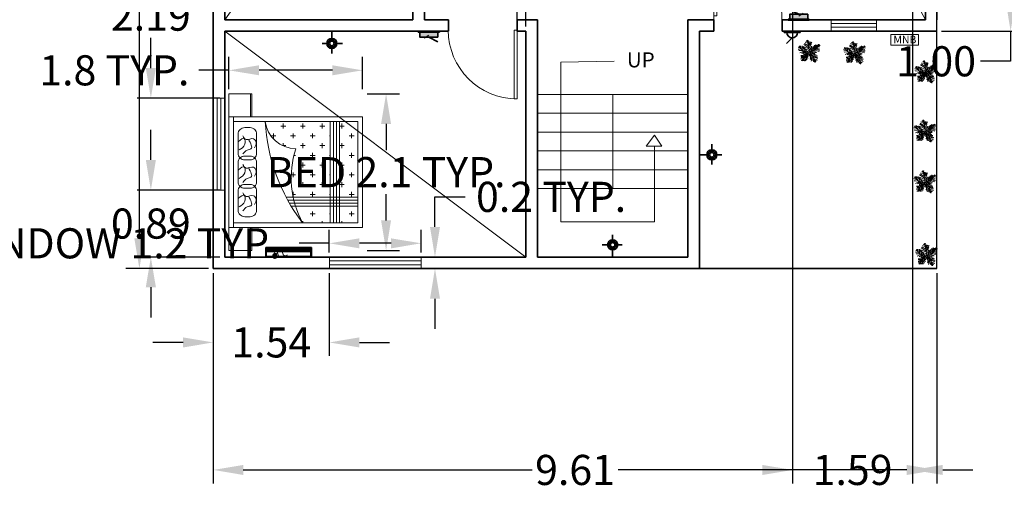
# Model space of a CAD drawing. Units: metres. Extents: x 24.2 to 58.5, y -14.5 to 15.2.
# Tile 4 of 7: x 38.9 to 51.9, y -1 to 5.2. Entities that reach past the tile are written whole.
import ezdxf

# ---------------------------------------------------------------- set-up
doc = ezdxf.new("R2010")
doc.units = ezdxf.units.M
doc.header["$MEASUREMENT"] = 0
for name, color, linetype, lineweight in [('A-ANNO-SYMB', 90, 'Continuous', 18), ('A-ANNO-TEXT', 10, 'Continuous', 18), ('A-FLOR', 7, 'Continuous', 25), ('A-FLOR-STRS', 7, 'Continuous', 18), ('A-GLAZ', 15, 'Continuous', 18), ('A-WALL', 7, 'Continuous', 35), ('DIMENSION', 90, 'Continuous', 18), ('DOOR', 15, 'Continuous', 18), ('E-COMM', 1, 'Continuous', 18), ('E-EQPM-LAYO', 1, 'Continuous', 13), ('E-LITE', 1, 'Continuous', 18), ('E-POWR', 1, 'Continuous', 18), ('E-POWR-EQPM', 1, 'Continuous', 18), ('Elec', 1, 'Continuous', 35), ('FURN', 163, 'Continuous', 13), ('L-PLNT', 90, 'Continuous', 13)]:
    doc.layers.add(name, color=color, linetype=linetype, lineweight=lineweight)
doc.styles.get("Standard").update_dxf_attribs({"font": 'arial.ttf'})
doc.dimstyles.get("Standard").update_dxf_attribs({"dimtxt": 0.4, "dimasz": 0.4, "dimexe": 0.18, "dimexo": 0.0625, "dimgap": 0.09, "dimtad": 0, "dimtih": 1, "dimtoh": 1, "dimdec": 1, "dimzin": 0, "dimdsep": 46, "dimtxsty": 'Standard', "dimcen": 0.09, "dimadec": 0, "dimazin": 0, "dimtfac": 1, "dimtdec": 1, "dimtofl": 0, "dimtmove": 0, "dimatfit": 3, "dimfxl": 1, "dimtolj": 1, "dimtzin": 0, "dimarcsym": 0})

# ---------------------------------------------------------------- blocks, each defined once
blk = doc.blocks.new('*U17')
for p, q in [((0, 0), (0, -6)), ((40, 0), (40, -6))]:
    blk.add_line(p, q)
blk.add_lwpolyline([(0, 0), (0, 40), (1.75, 40), (1.75, 0)], close=True)
blk.add_arc((0, 0), 40, 0, 90)
blk = doc.blocks.new('bed 1')
at = {"layer": 'FURN'}
h = blk.add_hatch(dxfattribs=at)
h.set_pattern_fill('CROSS', color=256, style=0)
h.set_pattern_definition([(0, (0, 0), (6.35, 6.35), [3.175, -9.525]), (90, (1.5875, -1.5875), (-6.35, 6.35), [3.175, -9.525])])
h.paths.add_polyline_path([(1334.16, -843.32, 0.37496), (1316.43, -863.27, 0.131129), (1284.95, -861.51), (1284.95, -885.72), (1334.16, -885.72)])
h.paths.add_polyline_path([(1278.95, -863.08, 0.048033), (1268.16, -867.67), (1268.16, -885.72), (1278.95, -885.72)])
h.paths.add_polyline_path([(1278.95, -891.72), (1268.16, -891.72), (1268.16, -903.72), (1278.95, -903.72)])
h.paths.add_polyline_path([(1334.16, -891.72), (1284.95, -891.72), (1284.95, -903.72), (1334.16, -903.72)])
for p, q in [((1265.16, -819.72), (1250.16, -819.72)), ((1250.16, -819.72), (1250.16, -834.72)), ((1337.16, -819.72), (1265.16, -819.72)), ((1265.16, -819.72), (1265.16, -906.72)), ((1337.16, -906.72), (1337.16, -819.72)), ((1337.16, -819.72), (1352.16, -819.72)), ((1352.16, -819.72), (1352.16, -834.72)), ((1337.16, -822.72), (1265.16, -822.72)), ((1268.16, -822.72), (1268.16, -903.72)), ((1334.16, -903.72), (1334.16, -822.72)), ((1250.16, -833.72), (1265.16, -833.72)), ((1250.16, -834.72), (1265.16, -834.72)), ((1352.16, -833.72), (1337.16, -833.72)), ((1352.16, -834.72), (1337.16, -834.72)), ((1282.95, -903.72), (1282.95, -857.98)), ((1284.95, -903.72), (1284.95, -856.89)), ((1278.95, -903.72), (1278.95, -860.29)), ((1280.95, -903.72), (1280.95, -859.11)), ((1334.16, -885.72), (1268.16, -885.72)), ((1334.16, -887.72), (1268.16, -887.72)), ((1334.16, -889.72), (1268.16, -889.72)), ((1334.16, -891.72), (1268.16, -891.72)), ((1268.16, -903.72), (1334.16, -903.72)), ((1265.16, -906.72), (1337.16, -906.72))]:
    blk.add_line(p, q, dxfattribs=at)
for points in [[(1288.91, -837.72), (1276.42, -837.72, -0.414214), (1272.16, -833.47), (1272.16, -829.98, -0.414214), (1276.42, -825.72), (1288.91, -825.72, -0.414214), (1293.16, -829.98), (1293.16, -833.47, -0.414214)], [(1307.41, -837.72), (1294.92, -837.72, -0.414214), (1290.66, -833.47), (1290.66, -829.98, -0.414214), (1294.92, -825.72), (1307.41, -825.72, -0.414214), (1311.66, -829.98), (1311.66, -833.47, -0.414214)], [(1325.91, -837.72), (1313.42, -837.72, -0.414214), (1309.16, -833.47), (1309.16, -829.98, -0.414214), (1313.42, -825.72), (1325.91, -825.72, -0.414214), (1330.16, -829.98), (1330.16, -833.47, -0.414214)], [(1334.16, -843.32, 0.151933), (1268.16, -867.67), (1268.16, -867.67, -0.20661), (1316.43, -863.27), (1316.43, -863.27, -0.37496)]]:
    blk.add_lwpolyline(points, format="xyb", close=True, dxfattribs=at)
for points, knots in [([(1278.62, -826.37), (1279.52, -827.92), (1281.07, -830.61), (1287.77, -830.3), (1285.41, -827.44), (1284.17, -825.93)], [0, 0, 0, 0, 4.23607, 7.317462, 10.761159, 10.761159, 10.761159, 10.761159]), ([(1297.12, -826.37), (1298.02, -827.92), (1299.57, -830.61), (1306.27, -830.3), (1303.91, -827.44), (1302.67, -825.93)], [0, 0, 0, 0, 4.23607, 7.317462, 10.761159, 10.761159, 10.761159, 10.761159]), ([(1315.62, -826.37), (1316.52, -827.92), (1318.07, -830.61), (1324.77, -830.3), (1322.41, -827.44), (1321.17, -825.93)], [0, 0, 0, 0, 4.23607, 7.317462, 10.761159, 10.761159, 10.761159, 10.761159]), ([(1275.98, -828.74), (1277, -829.54), (1278.71, -830.85), (1279.22, -835.95), (1282.92, -833.91), (1285.58, -832.44)], [0, 0, 0, 0, 3.079719, 5.108686, 10.317752, 10.317752, 10.317752, 10.317752]), ([(1287.7, -828.74), (1286.63, -829.38), (1283.96, -830.98), (1287.28, -835.52), (1283.18, -838.02), (1281.17, -836.99), (1280.03, -836.4)], [0, 0, 0, 0, 2.624379, 6.568207, 8.823918, 11.783788, 11.783788, 11.783788, 11.783788]), ([(1294.48, -828.74), (1295.5, -829.54), (1297.21, -830.85), (1297.72, -835.95), (1301.42, -833.91), (1304.08, -832.44)], [0, 0, 0, 0, 3.079719, 5.108686, 10.317752, 10.317752, 10.317752, 10.317752]), ([(1306.2, -828.74), (1305.13, -829.38), (1302.46, -830.98), (1305.78, -835.52), (1301.68, -838.02), (1299.67, -836.99), (1298.53, -836.4)], [0, 0, 0, 0, 2.624379, 6.568207, 8.823918, 11.783788, 11.783788, 11.783788, 11.783788]), ([(1312.98, -828.74), (1314, -829.54), (1315.71, -830.85), (1316.22, -835.95), (1319.92, -833.91), (1322.58, -832.44)], [0, 0, 0, 0, 3.079719, 5.108686, 10.317752, 10.317752, 10.317752, 10.317752]), ([(1324.7, -828.74), (1323.63, -829.38), (1320.96, -830.98), (1324.28, -835.52), (1320.18, -838.02), (1318.17, -836.99), (1317.03, -836.4)], [0, 0, 0, 0, 2.624379, 6.568207, 8.823918, 11.783788, 11.783788, 11.783788, 11.783788])]:
    blk.add_open_spline(points, degree=3, knots=knots, dxfattribs=at)
blk = doc.blocks.new('splight')
at = {"layer": 'Elec'}
for p, q in [((4618.17, 527.16), (4627.57, 527.16)), ((4622.87, 527.16), (4622.87, 523.87)), ((4620.58, 521.58), (4618.05, 521.58)), ((4625.16, 521.58), (4627.23, 521.58)), ((4622.87, 519.28), (4622.87, 517.03))]:
    blk.add_line(p, q, dxfattribs=at)
for radius in [2.29, 1.67, 1.04]:
    blk.add_circle((4622.87, 521.58), radius, dxfattribs=at)
blk = doc.blocks.new('BELL SWITCH')
at = {"layer": 'Elec'}
for p, q in [((4981.81, 3401.31), (4981.81, 3402.27)), ((4981.81, 3402.27), (4993.57, 3402.27)), ((4993.57, 3401.31), (4981.81, 3401.31)), ((4987.69, 3397.36), (4983.52, 3393.3)), ((4993.57, 3402.27), (4993.57, 3401.31))]:
    blk.add_line(p, q, dxfattribs=at)
blk.add_arc((4987.69, 3401.31), 3.95, 180, 0, dxfattribs=at)
blk = doc.blocks.new('*U44')
for p, q in [((-8.737, 47.138), (-17.069, 52.711)), ((-10.186, 53.64), (-13.084, 55.962)), ((0, 0), (-10.5, 57)), ((-9.099, 51.782), (-6.563, 55.962)), ((-7.65, 43.423), (-2.578, 49.46)), ((-5.839, 35.992), (4.667, 48.067)), ((-47.498, 19.737), (-55.83, 18.344)), ((-40.615, 13.7), (-55.105, 10.913)), ((-31.5, 4.5), (-52.5, 25.5)), ((-33.37, 6.269), (-52.207, 5.34)), ((-48.585, 21.131), (-49.309, 29.026)), ((-28.299, 3.483), (-47.86, -5.805)), ((-43.513, 28.561), (-42.427, 15.558)), ((-38.442, 26.239), (-34.819, 7.663)), ((-21.416, 3.018), (-38.079, -8.128)), ((-35.544, 28.097), (-24.314, 3.947)), ((0, 0), (-31.5, 4.5)), ((-14.533, 2.09), (-30.834, 25.31)), ((-15.982, 2.09), (-30.11, -9.521)), ((-3.665, 19.273), (-27.574, 35.527)), ((-5.114, 28.097), (-24.676, 40.636)), ((-24.314, 23.917), (-2.941, 13.7)), ((0, 0), (-22.5, -19.5)), ((-7.288, 39.707), (-21.778, 46.673)), ((-6.563, 1.161), (-21.416, -8.128)), ((-20.691, 13.7), (-1.129, 4.876)), ((-5.114, 27.632), (10.463, 46.673)), ((-2.941, 16.486), (8.652, 37.85)), ((-1.129, 6.734), (9.014, 26.704)), ((0, 0), (27, 9)), ((0, 0), (18, -22.5)), ((3.942, 1.625), (11.187, 24.381)), ((6.478, 1.625), (26.04, -8.592)), ((10.101, 3.483), (17.708, 26.239)), ((11.187, 3.483), (30.749, -5.805)), ((16.259, 5.805), (23.142, 31.348)), ((18.07, 5.805), (35.096, -3.483)), ((22.055, 7.198), (27.489, 32.277)), ((24.229, 7.663), (46.688, 1.625)), ((27, 9), (48, 36)), ((27.127, 9.056), (31.112, 35.992)), ((29.662, 12.307), (48.137, 6.269)), ((31.836, 30.883), (32.561, 16.486)), ((33.285, 16.486), (48.862, 10.913)), ((35.096, 32.741), (37.27, 22.524)), ((36.183, 19.737), (48.137, 17.88)), ((38.719, 34.134), (41.979, 28.561)), ((40.53, 25.775), (48.862, 24.846)), ((43.791, 29.954), (51.036, 30.883)), ((44.153, 36.456), (45.239, 32.741)), ((-17.431, -15.094), (-42.789, -18.809)), ((-28.299, -29.026), (-42.789, -31.348)), ((-24.314, -21.596), (-42.427, -22.06)), ((-30.834, -34.135), (-42.427, -35.528)), ((-34.457, -39.708), (-40.978, -42.494)), ((-26.849, -26.24), (-40.253, -25.775)), ((-22.5, -19.5), (-37.5, -45)), ((-32.646, -36.921), (-31.921, -44.352)), ((-15.257, -12.772), (-30.11, -12.772)), ((-29.023, -30.884), (-27.936, -43.887)), ((-25.038, -23.918), (-22.865, -45.281)), ((-20.691, -18.345), (-17.793, -44.352)), ((-6.563, -5.805), (-19.967, -9.985)), ((-17.069, -15.094), (-12.721, -40.172)), ((-13.446, -11.378), (-8.737, -32.741)), ((-9.461, -8.592), (-6.201, -23.453)), ((-4.752, -3.483), (-3.665, -14.629)), ((2.493, -3.019), (-1.491, -20.202)), ((1.769, -2.555), (24.229, -9.521)), ((5.029, -6.27), (2.131, -25.775)), ((9.014, -11.378), (3.58, -35.992)), ((14.085, -16.951), (6.478, -40.172)), ((7.565, -9.056), (32.198, -14.629)), ((18.07, -22.524), (8.289, -45.745)), ((12.274, -15.094), (36.907, -18.809)), ((20.244, -30.419), (15.897, -44.816)), ((16.259, -19.738), (36.183, -22.989)), ((18, -22.5), (27, -52.5)), ((18.433, -22.524), (40.53, -29.026)), ((19.157, -25.311), (38.719, -33.206)), ((22.78, -37.85), (19.519, -48.532)), ((21.331, -32.741), (39.081, -40.636)), ((22.78, -38.314), (34.372, -44.816)), ((24.591, -45.745), (23.142, -50.854)), ((24.591, -43.423), (30.749, -47.603)), ((26.764, -49.925), (28.213, -50.854))]:
    blk.add_line(p, q)
blk = doc.blocks.new('WINDOW-1220')
for p, q in [((0.152, 1.22), (0, 1.22)), ((0.051, 0), (0.051, 1.22)), ((0.102, 0), (0.102, 1.22)), ((0.152, 0), (0, 0))]:
    blk.add_line(p, q)
blk = doc.blocks.new('STAIR-FLIGHT-2000')
for p, q in [((0, 1.25), (2, 1.25)), ((0, 1), (2, 1)), ((0, 0.75), (2, 0.75)), ((0, 0.5), (2, 0.5)), ((0, 0.25), (2, 0.25)), ((0, 0), (2, 0))]:
    blk.add_line(p, q)
blk = doc.blocks.new('STAIR-PATH-UP')
for p, q in [((0.708, 2.134), (0, 2.121)), ((0, 2.121), (0, 0)), ((1.133, 1.007), (1.242, 1.15)), ((1.242, 1.15), (1.342, 1.007)), ((1.242, 1.007), (1.133, 1.007)), ((1.242, 0), (1.242, 1.007)), ((1.342, 1.007), (1.242, 1.007)), ((0, 0), (1.242, 0))]:
    blk.add_line(p, q)
blk = doc.blocks.new('MAIN-BOARD-TAG')
blk.add_lwpolyline([(0, 0.142), (0.366, 0.142), (0.366, 0), (0, 0)], close=True)
blk.add_text('MNB', height=0.102).set_placement((0.035, 0.024))
blk = doc.blocks.new('elec box')
at = {"layer": 'Elec'}
blk.add_hatch(color=256, dxfattribs=at).paths.add_polyline_path([(3828.23, 599.29), (3828.23, 594.79), (3844.73, 594.79), (3844.73, 599.29)])
for p, q in [((3836.48, 599.29), (3828.07, 603.45)), ((3846.1, 594.79), (3826.83, 594.79)), ((3826.83, 594.79), (3826.83, 593.89)), ((3826.83, 593.89), (3846.1, 593.89)), ((3846.1, 593.89), (3846.1, 594.79))]:
    blk.add_line(p, q, dxfattribs=at)
blk.add_lwpolyline([(3828.23, 594.79), (3828.23, 599.29), (3844.73, 599.29), (3844.73, 594.79), (3828.23, 594.79)], dxfattribs=at)
blk = doc.blocks.new('SWITCHBOARD-ONE-WAY')
blk.add_line((0.14, 0.052), (0.201, 0.094))
at = {"xscale": 0.0145668999005024, "yscale": 0.0145668999005024, "zscale": 0.0145668999005024}
blk.add_blockref('elec box', (-55.745, -8.651), dxfattribs=at)
blk = doc.blocks.new('ac')
at = {"layer": 'Elec'}
for p, q in [((12718.34, -53.78), (12674.36, -53.78)), ((12674.36, -63.02), (12674.36, -53.78)), ((12675.81, -57.52), (12675.81, -53.78)), ((12717.03, -54.85), (12675.81, -54.85)), ((12717.03, -56.21), (12675.81, -56.21)), ((12717.03, -57.52), (12717.03, -53.78)), ((12718.34, -63.02), (12718.34, -53.78)), ((12718.34, -63.02), (12674.36, -63.02)), ((12674.89, -57.52), (12717.81, -57.52))]:
    blk.add_line(p, q, dxfattribs=at)
at = {"layer": 'Elec', "ltscale": 0.1}
for p, q in [((12674.89, -61.49), (12674.89, -53.78)), ((12717.03, -54.36), (12675.81, -54.36)), ((12717.03, -55.66), (12675.81, -55.66)), ((12717.03, -56.84), (12675.81, -56.84)), ((12717.81, -61.49), (12717.81, -53.78)), ((12716.81, -62.49), (12675.89, -62.49))]:
    blk.add_line(p, q, dxfattribs=at)
at = {"layer": 'Elec'}
for centre, start, end in [((12675.89, -61.49), 180, 270), ((12716.81, -61.49), 270, 0)]:
    blk.add_arc(centre, 1, start, end, dxfattribs=at)
blk = doc.blocks.new('AC-POINT-LABELED')
at = {"xscale": 0.0137983327653967, "yscale": 0.0137983327653967, "zscale": 0.0137983327653967}
blk.add_blockref('ac', (-174.885, 0.87), dxfattribs=at)
blk.add_text(' A C', height=0.102).set_placement((0.062, 0.014))
blk = doc.blocks.new('*D57')
at = {"layer": 'Defpoints', "color": 0, "transparency": 16777216}
for p in [(43.407, 4.217), (43.719, 4.217), (43.407, 2.137)]:
    blk.add_point(p, dxfattribs=at)
at = {"layer": 'DIMENSION', "color": 0, "lineweight": -2, "transparency": 16777216}
for p, q in [((43.469, 4.217), (43.899, 4.217)), ((43.719, 3.817), (43.719, 3.468)), ((43.719, 2.537), (43.719, 2.886)), ((43.469, 2.137), (43.899, 2.137))]:
    blk.add_line(p, q, dxfattribs=at)
at = {"layer": 'DIMENSION', "color": 0, "transparency": 16777216}
for points in [[(43.652, 3.817), (43.785, 3.817), (43.719, 4.217)], [(43.652, 2.537), (43.785, 2.537), (43.719, 2.137)]]:
    blk.add_solid(points, dxfattribs=at)
at = {"layer": 'DIMENSION', "color": 0, "transparency": 16777216, "insert": (43.719, 3.177), "char_height": 0.4, "attachment_point": 5}
blk.add_mtext('\\A1;BED 2.1 TYP.', dxfattribs=at)
blk = doc.blocks.new('*D58')
at = {"layer": 'Defpoints', "color": 0, "transparency": 16777216}
for p in [(41.632, 4.529), (41.632, 4.217), (43.407, 4.217)]:
    blk.add_point(p, dxfattribs=at)
at = {"layer": 'DIMENSION', "color": 0, "lineweight": -2, "transparency": 16777216}
for p, q in [((41.632, 4.28), (41.632, 4.709)), ((43.407, 4.28), (43.407, 4.709)), ((41.632, 4.529), (41.232, 4.529)), ((43.007, 4.529), (42.032, 4.529))]:
    blk.add_line(p, q, dxfattribs=at)
at = {"layer": 'DIMENSION', "color": 0, "transparency": 16777216}
for points in [[(42.032, 4.596), (42.032, 4.463), (41.632, 4.529)], [(43.007, 4.596), (43.007, 4.463), (43.407, 4.529)]]:
    blk.add_solid(points, dxfattribs=at)
at = {"layer": 'DIMENSION', "color": 0, "transparency": 16777216, "insert": (40.11, 4.529), "char_height": 0.4, "attachment_point": 5}
blk.add_mtext('\\A1;1.8 TYP.', dxfattribs=at)
blk = doc.blocks.new('*D61')
at = {"layer": 'Defpoints', "color": 0, "transparency": 16777216}
for p in [(42.965, 2.232), (42.965, 2.049), (44.185, 2.049)]:
    blk.add_point(p, dxfattribs=at)
at = {"layer": 'DIMENSION', "color": 0, "lineweight": -2, "transparency": 16777216}
for p, q in [((42.965, 2.111), (42.965, 2.412)), ((44.185, 2.111), (44.185, 2.412)), ((42.965, 2.232), (42.565, 2.232)), ((43.785, 2.232), (43.365, 2.232))]:
    blk.add_line(p, q, dxfattribs=at)
at = {"layer": 'DIMENSION', "color": 0, "transparency": 16777216}
for points in [[(43.365, 2.298), (43.365, 2.165), (42.965, 2.232)], [(43.785, 2.298), (43.785, 2.165), (44.185, 2.232)]]:
    blk.add_solid(points, dxfattribs=at)
at = {"layer": 'DIMENSION', "color": 0, "transparency": 16777216, "insert": (40.113, 2.232), "char_height": 0.4, "attachment_point": 5}
blk.add_mtext('\\A1;WINDOW 1.2 TYP.', dxfattribs=at)
blk = doc.blocks.new('*D62')
at = {"layer": 'Defpoints', "color": 0, "transparency": 16777216}
for p in [(44.185, 2.049), (44.368, 2.049), (44.185, 1.896)]:
    blk.add_point(p, dxfattribs=at)
at = {"layer": 'DIMENSION', "color": 0, "lineweight": -2, "transparency": 16777216}
for p, q in [((44.368, 2.449), (44.368, 2.849)), ((44.368, 2.849), (44.768, 2.849)), ((44.248, 2.049), (44.548, 2.049)), ((44.248, 1.896), (44.548, 1.896)), ((44.368, 1.496), (44.368, 1.096))]:
    blk.add_line(p, q, dxfattribs=at)
at = {"layer": 'DIMENSION', "color": 0, "transparency": 16777216}
for points in [[(44.302, 2.449), (44.435, 2.449), (44.368, 2.049)], [(44.302, 1.496), (44.435, 1.496), (44.368, 1.896)]]:
    blk.add_solid(points, dxfattribs=at)
at = {"layer": 'DIMENSION', "color": 0, "transparency": 16777216, "insert": (45.91, 2.849), "char_height": 0.4, "attachment_point": 5}
blk.add_mtext('\\A1;0.2 TYP.', dxfattribs=at)
blk = doc.blocks.new('*D107')
at = {"layer": 'Defpoints', "color": 0, "transparency": 16777216}
for p in [(41.423, 1.896), (51.033, 1.896), (41.423, -0.777)]:
    blk.add_point(p, dxfattribs=at)
at = {"layer": 'DIMENSION', "color": 0, "lineweight": -2, "transparency": 16777216}
for p, q in [((41.423, 1.834), (41.423, -0.957)), ((51.033, 1.834), (51.033, -0.957)), ((41.823, -0.777), (45.657, -0.777)), ((50.633, -0.777), (46.799, -0.777))]:
    blk.add_line(p, q, dxfattribs=at)
at = {"layer": 'DIMENSION', "color": 0, "transparency": 16777216}
for points in [[(41.823, -0.711), (41.823, -0.844), (41.423, -0.777)], [(50.633, -0.711), (50.633, -0.844), (51.033, -0.777)]]:
    blk.add_solid(points, dxfattribs=at)
at = {"layer": 'DIMENSION', "color": 0, "transparency": 16777216, "insert": (46.228, -0.777), "char_height": 0.4, "attachment_point": 5}
blk.add_mtext('\\A1;9.61', dxfattribs=at)
blk = doc.blocks.new('*D108')
at = {"layer": 'Defpoints', "color": 0, "transparency": 16777216}
for p in [(40.443, 13.506), (44.075, 13.506), (41.423, 1.896)]:
    blk.add_point(p, dxfattribs=at)
at = {"layer": 'DIMENSION', "color": 0, "lineweight": -2, "transparency": 16777216}
for p, q in [((44.013, 13.506), (40.263, 13.506)), ((40.443, 13.106), (40.443, 7.995)), ((40.443, 2.296), (40.443, 7.407)), ((41.361, 1.896), (40.263, 1.896))]:
    blk.add_line(p, q, dxfattribs=at)
at = {"layer": 'DIMENSION', "color": 0, "transparency": 16777216}
for points in [[(40.376, 13.106), (40.509, 13.106), (40.443, 13.506)], [(40.376, 2.296), (40.509, 2.296), (40.443, 1.896)]]:
    blk.add_solid(points, dxfattribs=at)
at = {"layer": 'DIMENSION', "color": 0, "transparency": 16777216, "insert": (40.443, 7.701), "char_height": 0.4, "attachment_point": 5}
blk.add_mtext('\\A1;11.61', dxfattribs=at)
blk = doc.blocks.new('*D109')
at = {"layer": 'Defpoints', "color": 0, "transparency": 16777216}
for p in [(40.595, 2.939), (41.575, 2.939), (41.575, 2.049)]:
    blk.add_point(p, dxfattribs=at)
at = {"layer": 'DIMENSION', "color": 0, "lineweight": -2, "transparency": 16777216}
for p, q in [((40.595, 3.339), (40.595, 3.739)), ((41.513, 2.939), (40.415, 2.939)), ((41.513, 2.049), (40.415, 2.049)), ((40.595, 1.649), (40.595, 1.249))]:
    blk.add_line(p, q, dxfattribs=at)
at = {"layer": 'DIMENSION', "color": 0, "transparency": 16777216}
for points in [[(40.528, 3.339), (40.662, 3.339), (40.595, 2.939)], [(40.528, 1.649), (40.662, 1.649), (40.595, 2.049)]]:
    blk.add_solid(points, dxfattribs=at)
at = {"layer": 'DIMENSION', "color": 0, "transparency": 16777216, "insert": (40.595, 2.494), "char_height": 0.4, "attachment_point": 5}
blk.add_mtext('\\A1;0.89', dxfattribs=at)
blk = doc.blocks.new('*D110')
at = {"layer": 'Defpoints', "color": 0, "transparency": 16777216}
for p in [(40.595, 6.351), (41.575, 6.351), (41.575, 4.159)]:
    blk.add_point(p, dxfattribs=at)
at = {"layer": 'DIMENSION', "color": 0, "lineweight": -2, "transparency": 16777216}
for p, q in [((41.513, 6.351), (40.415, 6.351)), ((40.595, 5.951), (40.595, 5.549)), ((40.595, 4.559), (40.595, 4.961)), ((41.513, 4.159), (40.415, 4.159))]:
    blk.add_line(p, q, dxfattribs=at)
at = {"layer": 'DIMENSION', "color": 0, "transparency": 16777216}
for points in [[(40.528, 5.951), (40.662, 5.951), (40.595, 6.351)], [(40.528, 4.559), (40.662, 4.559), (40.595, 4.159)]]:
    blk.add_solid(points, dxfattribs=at)
at = {"layer": 'DIMENSION', "color": 0, "transparency": 16777216, "insert": (40.595, 5.255), "char_height": 0.4, "attachment_point": 5}
blk.add_mtext('\\A1;2.19', dxfattribs=at)
blk = doc.blocks.new('*D113')
at = {"layer": 'Defpoints', "color": 0, "transparency": 16777216}
for p in [(51.033, 6.048), (51.033, 5.049), (52.013, 5.049)]:
    blk.add_point(p, dxfattribs=at)
at = {"layer": 'DIMENSION', "color": 0, "lineweight": -2, "transparency": 16777216}
for p, q in [((51.095, 6.048), (52.193, 6.048)), ((52.013, 5.648), (52.013, 5.449)), ((51.095, 5.049), (52.193, 5.049)), ((52.013, 5.049), (52.013, 4.649)), ((52.013, 4.649), (51.613, 4.649))]:
    blk.add_line(p, q, dxfattribs=at)
at = {"layer": 'DIMENSION', "color": 0, "transparency": 16777216}
for points in [[(51.947, 5.648), (52.08, 5.648), (52.013, 6.048)], [(51.947, 5.449), (52.08, 5.449), (52.013, 5.049)]]:
    blk.add_solid(points, dxfattribs=at)
at = {"layer": 'DIMENSION', "color": 0, "transparency": 16777216, "insert": (51.023, 4.649), "char_height": 0.4, "attachment_point": 5}
blk.add_mtext('\\A1;1.00', dxfattribs=at)
blk = doc.blocks.new('*D116')
at = {"layer": 'Defpoints', "color": 0, "transparency": 16777216}
for p in [(41.423, 1.896), (42.965, 1.896), (41.423, 0.916)]:
    blk.add_point(p, dxfattribs=at)
at = {"layer": 'DIMENSION', "color": 0, "lineweight": -2, "transparency": 16777216}
for p, q in [((41.423, 1.834), (41.423, 0.736)), ((42.965, 1.834), (42.965, 0.736)), ((41.023, 0.916), (40.623, 0.916)), ((43.365, 0.916), (43.765, 0.916))]:
    blk.add_line(p, q, dxfattribs=at)
at = {"layer": 'DIMENSION', "color": 0, "transparency": 16777216}
for points in [[(41.023, 0.983), (41.023, 0.849), (41.423, 0.916)], [(43.365, 0.983), (43.365, 0.849), (42.965, 0.916)]]:
    blk.add_solid(points, dxfattribs=at)
at = {"layer": 'DIMENSION', "color": 0, "transparency": 16777216, "insert": (42.194, 0.916), "char_height": 0.4, "attachment_point": 5}
blk.add_mtext('\\A1;1.54', dxfattribs=at)
blk = doc.blocks.new('*D119')
at = {"layer": 'Defpoints', "color": 0, "transparency": 16777216}
for p in [(49.117, 6.114), (50.711, 6.114), (50.711, -0.777)]:
    blk.add_point(p, dxfattribs=at)
at = {"layer": 'DIMENSION', "color": 0, "lineweight": -2, "transparency": 16777216}
for p, q in [((49.117, 6.051), (49.117, -0.957)), ((50.711, 6.051), (50.711, -0.957)), ((48.717, -0.777), (48.317, -0.777)), ((51.111, -0.777), (51.511, -0.777))]:
    blk.add_line(p, q, dxfattribs=at)
at = {"layer": 'DIMENSION', "color": 0, "transparency": 16777216}
for points in [[(48.717, -0.711), (48.717, -0.844), (49.117, -0.777)], [(51.111, -0.711), (51.111, -0.844), (50.711, -0.777)]]:
    blk.add_solid(points, dxfattribs=at)
at = {"layer": 'DIMENSION', "color": 0, "transparency": 16777216, "insert": (49.914, -0.777), "char_height": 0.4, "attachment_point": 5}
blk.add_mtext('\\A1;1.59', dxfattribs=at)
blk = doc.blocks.new('*D125')
at = {"layer": 'Defpoints', "color": 0, "transparency": 16777216}
for p in [(45.575, 6.029), (45.459, 5.049), (45.575, 5.049)]:
    blk.add_point(p, dxfattribs=at)
at = {"layer": 'DIMENSION', "color": 0, "lineweight": -2, "transparency": 16777216}
for p, q in [((45.459, 5.111), (45.459, 6.209)), ((45.575, 5.111), (45.575, 6.209)), ((45.059, 6.029), (44.659, 6.029)), ((45.975, 6.029), (46.375, 6.029))]:
    blk.add_line(p, q, dxfattribs=at)
at = {"layer": 'DIMENSION', "color": 0, "transparency": 16777216}
for points in [[(45.059, 6.096), (45.059, 5.963), (45.459, 6.029)], [(45.975, 6.096), (45.975, 5.963), (45.575, 6.029)]]:
    blk.add_solid(points, dxfattribs=at)
at = {"layer": 'DIMENSION', "color": 0, "transparency": 16777216, "insert": (46.983, 6.029), "char_height": 0.4, "attachment_point": 5}
blk.add_mtext('\\A1;0.12', dxfattribs=at)

msp = doc.modelspace()

# ---------------------------------------------------------------- linework, layer by layer
at = {"layer": 'A-FLOR'}
msp.add_line((51.0327, 1.8964), (51.0327, 5.2012), dxfattribs=at)
at = {"layer": 'A-FLOR-STRS'}
msp.add_line((46.7279, 2.9588), (46.7279, 4.2088), dxfattribs=at)
at = {"layer": 'A-GLAZ'}
for p, q in [((49.63, 5.2012), (49.63, 5.0488)), ((50.23, 5.149), (49.63, 5.149)), ((50.23, 5.101), (49.63, 5.101)), ((50.23, 5.2012), (50.23, 5.0488))]:
    msp.add_line(p, q, dxfattribs=at)
at = {"layer": 'A-WALL'}
for p, q in [((41.4231, 1.8964), (41.4231, 10.3536)), ((51.0327, 5.2012), (51.0327, 10.3536)), ((50.8803, 5.2012), (50.8803, 10.2012)), ((41.5755, 5.2012), (41.5755, 8.7012)), ((44.0755, 5.2012), (44.0755, 7.6158)), ((44.2279, 5.2012), (44.2279, 7.6158)), ((41.5755, 5.2012), (44.0755, 5.2012)), ((44.2279, 5.2012), (44.5489, 5.2012)), ((44.5489, 5.0488), (44.5489, 5.2012)), ((45.4589, 5.0488), (45.4589, 5.2012)), ((45.4589, 5.2012), (45.7279, 5.2012)), ((45.7279, 2.0488), (45.7279, 5.2012)), ((47.7279, 5.2012), (48.0698, 5.2012)), ((47.7279, 2.0488), (47.7279, 5.2012)), ((48.0698, 5.0488), (48.0698, 5.2012)), ((48.9798, 5.0488), (48.9798, 5.2012)), ((48.9798, 5.2012), (50.8803, 5.2012)), ((41.5755, 5.0488), (44.5489, 5.0488)), ((41.5755, 2.0488), (41.5755, 5.0488)), ((45.4589, 5.0488), (45.5755, 5.0488)), ((45.5755, 2.0488), (45.5755, 5.0488)), ((47.8803, 5.0488), (48.0698, 5.0488)), ((47.8803, 1.8964), (47.8803, 5.0488)), ((48.9798, 5.0488), (51.0327, 5.0488)), ((41.5755, 2.0488), (45.5755, 2.0488)), ((45.7279, 2.0488), (47.7279, 2.0488)), ((41.4231, 1.8964), (51.0327, 1.8964))]:
    msp.add_line(p, q, dxfattribs=at)
at = {"layer": 'E-EQPM-LAYO'}
for p, q in [((50.8803, 5.2012), (48.2279, 10.2012)), ((41.5755, 5.2012), (44.0755, 8.7012)), ((41.5755, 5.0488), (45.5755, 2.0488))]:
    msp.add_line(p, q, dxfattribs=at)

# ---------------------------------------------------------------- block references
at = {"layer": 'A-ANNO-SYMB'}
msp.add_blockref('STAIR-PATH-UP', (46.0398, 2.517), dxfattribs=at)
at = {"layer": 'A-FLOR-STRS'}
msp.add_blockref('STAIR-FLIGHT-2000', (45.7281, 2.959), dxfattribs=at)
at = {"layer": 'A-GLAZ'}
msp.add_blockref('WINDOW-1220', (41.423, 2.939), dxfattribs=at)
at = {"layer": 'A-GLAZ', "rotation": 89.9999999999994}
msp.add_blockref('WINDOW-1220', (44.1853, 1.8963), dxfattribs=at)
at = {"layer": 'DOOR', "xscale": 0.0226094875306225, "yscale": 0.0226094875306225, "zscale": 0.0226094875306225}
msp.add_blockref('*U17', (48.0698, 5.2523), dxfattribs=at)
at = {"layer": 'DOOR', "xscale": 0.022862310694534, "yscale": 0.022862310694534, "zscale": 0.022862310694534, "rotation": 180}
msp.add_blockref('*U17', (45.4589, 5.0641), dxfattribs=at)
at = {"layer": 'E-COMM', "xscale": 0.0182086248757497, "yscale": 0.0182086248757497, "zscale": 0.0182086248757497}
msp.add_blockref('BELL SWITCH', (-41.707, -56.9018), dxfattribs=at)
at = {"layer": 'E-LITE', "xscale": -0.0291629336008972, "yscale": 0.0291629336008972, "zscale": 0.0291629336007624}
for p, rotation in [((177.8155, -10.3247), 359.9999999999997), ((63.2553, 138.2234), 89.99999999999969), ((-88.0886, 17.4223), 180)]:
    msp.add_blockref('splight', p, dxfattribs=dict(at, rotation=rotation))
at = {"layer": 'E-POWR'}
for name, p in [('SWITCHBOARD-ONE-WAY', (49.0588, 5.1944)), ('MAIN-BOARD-TAG', (50.4213, 4.8623))]:
    msp.add_blockref(name, p, dxfattribs=at)
at = {"layer": 'E-POWR', "rotation": 180}
msp.add_blockref('SWITCHBOARD-ONE-WAY', (44.4261, 5.0485), dxfattribs=at)
at = {"layer": 'E-POWR-EQPM'}
msp.add_blockref('AC-POINT-LABELED', (42.1204, 2.0487), dxfattribs=at)
at = {"layer": 'FURN', "xscale": 0.0203972636680773, "yscale": 0.0203972636680773, "zscale": 0.0203972636680773, "rotation": 90}
msp.add_blockref('bed 1', (24.912, -23.3632), dxfattribs=at)
at = {"layer": 'L-PLNT', "xscale": 0.0027252779435763, "yscale": 0.0027252779435763, "zscale": 0.0027252779435763}
for p in [(49.343, 4.7759), (49.343, 4.7759), (49.9464, 4.7559), (50.8912, 4.503), (50.8806, 3.7165), (50.8799, 3.0424), (50.901, 2.0766)]:
    msp.add_blockref('*U44', p, dxfattribs=at)

# ---------------------------------------------------------------- texts
at = {"layer": 'A-ANNO-TEXT', "insert": (46.9162, 4.768), "char_height": 0.2, "attachment_point": 1}
msp.add_mtext_dynamic_manual_height_columns('UP', width=0.350048, gutter_width=1, heights=[0], dxfattribs=at)

# ---------------------------------------------------------------- dimensions: what is measured, and where the dimension line sits
at = {"layer": 'DIMENSION'}
for base, p1, p2, angle, picture, middle in [((40.4426, 13.506), (41.4231, 1.8964), (44.0755, 13.506), 90, '*D108', (40.4426, 7.7012)), ((40.595, 6.3512), (41.5755, 4.1588), (41.5755, 6.3512), 90, '*D110', (40.595, 5.255)), ((52.0132, 5.0488), (51.0327, 6.0481), (51.0327, 5.0488), 270, '*D113', (51.0232, 4.6488)), ((40.595, 2.9388), (41.5755, 2.0488), (41.5755, 2.9388), 90, '*D109', (40.595, 2.4938)), ((41.4231, 0.9159), (42.9655, 1.8964), (41.4231, 1.8964), 180, '*D116', (42.1943, 0.9159))]:
    dim = msp.add_linear_dim(base=base, p1=p1, p2=p2, angle=angle, dimstyle='Standard', override={"dimdec": 2, "dimlfac": 1, "dimrnd": 0, "dimzin": 0, "dimdsep": 46, "dimlunit": 2}, dxfattribs=at)
    dim.commit()
    dim.dimension.update_dxf_attribs({"geometry": picture, "text_midpoint": middle})
for base, p1, p2, picture, middle in [((45.5755, 6.0293), (45.4589, 5.0488), (45.5755, 5.0488), '*D125', (46.9829, 6.0293)), ((50.7111, -0.7772), (49.1166, 6.114), (50.7111, 6.114), '*D119', (49.9138, -0.7772)), ((41.4231, -0.7772), (51.0327, 1.8964), (41.4231, 1.8964), '*D107', (46.2279, -0.7772))]:
    dim = msp.add_linear_dim(base=base, p1=p1, p2=p2, dimstyle='Standard', override={"dimdec": 2, "dimlfac": 1, "dimrnd": 0, "dimzin": 0, "dimdsep": 46, "dimlunit": 2}, dxfattribs=at)
    dim.commit()
    dim.dimension.update_dxf_attribs({"geometry": picture, "text_midpoint": middle})
for base, p1, p2, angle, text, picture, middle in [((41.6321, 4.5293), (43.4067, 4.2172), (41.6321, 4.2172), 180, '<> TYP.', '*D58', (40.1098, 4.5293)), ((43.7188, 4.2172), (43.4067, 2.1367), (43.4067, 4.2172), 90, 'BED <> TYP.', '*D57', (43.7188, 3.177)), ((44.3685, 2.0488), (44.1855, 1.8964), (44.1855, 2.0488), 90, '<> TYP.', '*D62', (45.9096, 2.8488)), ((42.9655, 2.2318), (44.1855, 2.0488), (42.9655, 2.0488), 180, 'WINDOW <> TYP.', '*D61', (40.1126, 2.2318))]:
    dim = msp.add_linear_dim(base=base, p1=p1, p2=p2, angle=angle, text=text, dimstyle='Standard', override={"dimdec": 1, "dimlfac": 1, "dimrnd": 0, "dimzin": 0, "dimdsep": 46, "dimlunit": 2}, dxfattribs=at)
    dim.commit()
    dim.dimension.update_dxf_attribs({"geometry": picture, "text_midpoint": middle})

doc.saveas('drawing.dxf')
